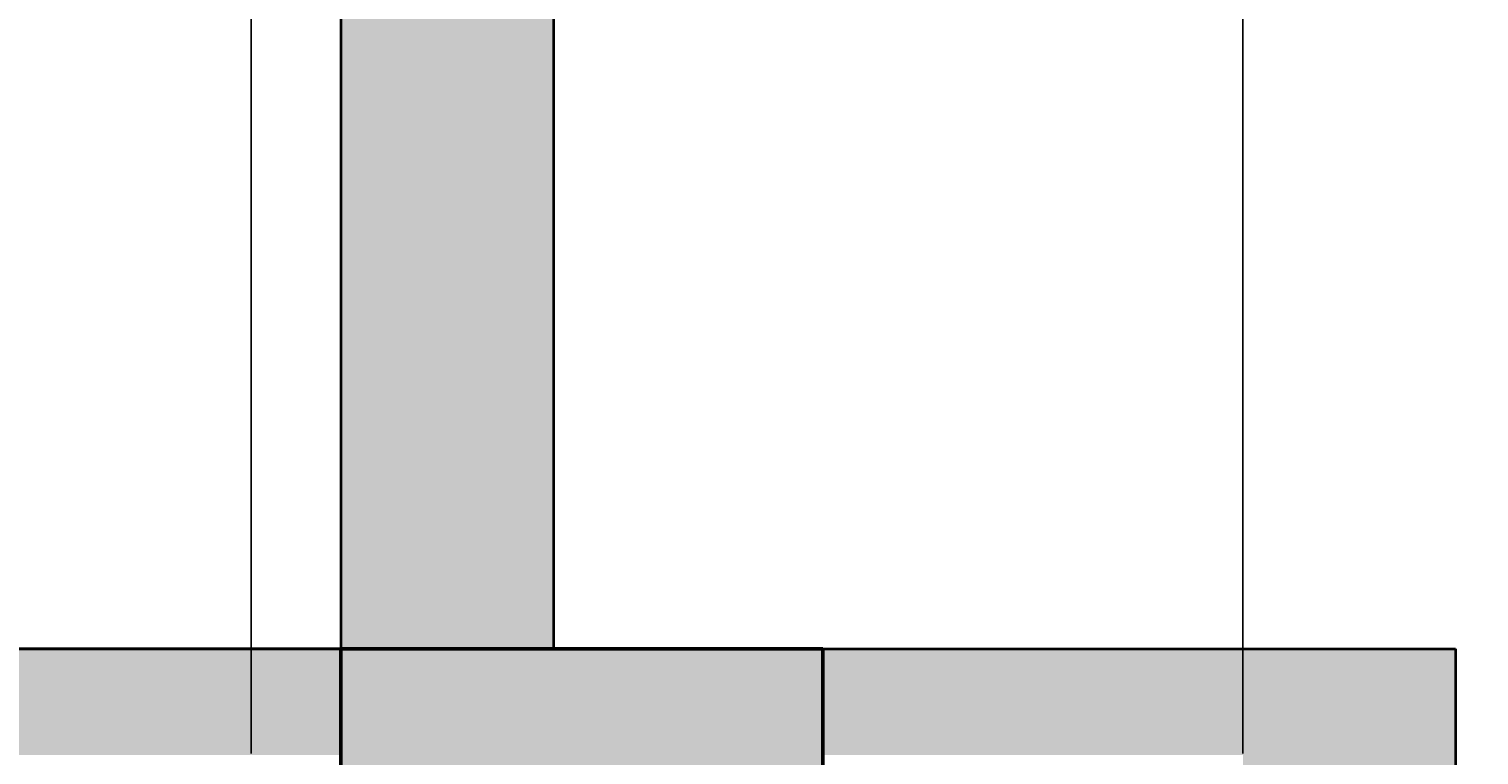
# Model space of a CAD drawing. Units: inches. Extents: x 1998 to 2588, y 1139 to 1977.
# Tile 130 of 134: x 2489 to 2550, y 1637 to 1667. Entities that reach past the tile are written whole.
import ezdxf

# ---------------------------------------------------------------- set-up
doc = ezdxf.new("R2010")
doc.units = ezdxf.units.IN
for name, color, linetype, lineweight in [('A-ANNO-DIMS', 2, 'Continuous', 18), ('A-COLS-PATT', 250, 'Continuous', 13), ('A-WALL-PATT', 252, 'Continuous', 13), ('COLUMN', 10, 'Continuous', 50), ('WALL', 200, 'Continuous', 35)]:
    doc.layers.add(name, color=color, linetype=linetype, lineweight=lineweight)
doc.styles.get("Standard").update_dxf_attribs({"font": 'arial.ttf'})
doc.dimstyles.get("Standard").update_dxf_attribs({"dimtxt": 0.18, "dimasz": 0.18, "dimexe": 0.18, "dimexo": 0.0625, "dimgap": 0.09, "dimtad": 0, "dimtih": 1, "dimtoh": 1, "dimdec": 4, "dimzin": 0, "dimdsep": 46, "dimtxsty": 'Standard', "dimcen": 0.09, "dimadec": 0, "dimazin": 0, "dimtfac": 1, "dimtdec": 4, "dimtofl": 0, "dimtmove": 0, "dimatfit": 3, "dimfxl": 1, "dimtolj": 1, "dimtzin": 0, "dimarcsym": 0})

# ---------------------------------------------------------------- blocks, each defined once
blk = doc.blocks.new('*D24')
at = {"layer": 'A-ANNO-DIMS', "color": 0, "lineweight": -2, "transparency": 16777216}
for p, q in [((2398.535, 1911.232), (2588.309, 1911.232)), ((2588.129, 1911.052), (2588.129, 1570.164)), ((2588.129, 1228.912), (2588.129, 1569.8)), ((2527.535, 1228.732), (2588.309, 1228.732))]:
    blk.add_line(p, q, dxfattribs=at)
at = {"layer": 'A-ANNO-DIMS', "color": 0, "transparency": 16777216}
for points in [[(2588.099, 1911.052), (2588.159, 1911.052), (2588.129, 1911.232)], [(2588.099, 1228.912), (2588.159, 1228.912), (2588.129, 1228.732)]]:
    blk.add_solid(points, dxfattribs=at)
at = {"layer": 'Defpoints', "color": 0, "transparency": 16777216}
for p in [(2398.473, 1911.232), (2588.129, 1911.232), (2527.473, 1228.732)]:
    blk.add_point(p, dxfattribs=at)
at = {"layer": 'A-ANNO-DIMS', "color": 0, "transparency": 16777216, "insert": (2588.129, 1569.982), "char_height": 0.18, "attachment_point": 5}
blk.add_mtext('\\A1;682.5', dxfattribs=at)
blk = doc.blocks.new('*D31')
at = {"layer": 'A-ANNO-DIMS', "color": 0, "lineweight": -2, "transparency": 16777216}
for p, q in [((2498.179, 1636.795), (2498.179, 1977.362)), ((2498.359, 1977.182), (2518.957, 1977.182)), ((2539.999, 1977.182), (2519.4, 1977.182)), ((2540.179, 1636.795), (2540.179, 1977.362))]:
    blk.add_line(p, q, dxfattribs=at)
at = {"layer": 'A-ANNO-DIMS', "color": 0, "transparency": 16777216}
for points in [[(2498.359, 1977.212), (2498.359, 1977.152), (2498.179, 1977.182)], [(2539.999, 1977.212), (2539.999, 1977.152), (2540.179, 1977.182)]]:
    blk.add_solid(points, dxfattribs=at)
at = {"layer": 'Defpoints', "color": 0, "transparency": 16777216}
for p in [(2540.179, 1977.182), (2498.179, 1636.732), (2540.179, 1636.732)]:
    blk.add_point(p, dxfattribs=at)
at = {"layer": 'A-ANNO-DIMS', "color": 0, "transparency": 16777216, "insert": (2519.179, 1977.182), "char_height": 0.18, "attachment_point": 5}
blk.add_mtext('\\A1;42', dxfattribs=at)

msp = doc.modelspace()

# ---------------------------------------------------------------- hatches: boundary and pattern name
at = {"layer": 'A-COLS-PATT'}
h = msp.add_hatch(color=256, dxfattribs=at)
h.dxf.hatch_style = 1
h.paths.add_polyline_path([(2099.4125, 1888.7324), (2087.9729, 1888.7324), (2087.9729, 1868.3278), (2099.4125, 1868.3278)])
h.paths.add_polyline_path([(2234.4125, 1888.7324), (2222.9729, 1888.7324), (2222.9729, 1868.3278), (2234.4125, 1868.3278)])
h.paths.add_polyline_path([(2341.4729, 1886.637), (2330.0332, 1886.637), (2330.0332, 1866.2324), (2341.4729, 1866.2324)])
h.paths.add_polyline_path([(2507.8006, 1882.7324), (2487.396, 1882.7324), (2487.396, 1871.2927), (2507.8006, 1871.2927)])
h.paths.add_polyline_path([(2510.9729, 1766.672), (2490.5682, 1766.672), (2490.5682, 1755.2324), (2510.9729, 1755.2324)])
h.paths.add_polyline_path([(2345.9729, 1759.7324), (2334.5332, 1759.7324), (2334.5332, 1739.3278), (2345.9729, 1739.3278)])
h.paths.add_polyline_path([(2234.4125, 1774.3318), (2222.9729, 1774.3318), (2222.9729, 1753.9272), (2234.4125, 1753.9272)])
h.paths.add_polyline_path([(2099.4125, 1775.637), (2087.9729, 1775.637), (2087.9729, 1755.2324), (2099.4125, 1755.2324)])
h.paths.add_polyline_path([(2098.0956, 1593.7241), (2077.691, 1593.7241), (2077.691, 1582.2845), (2098.0956, 1582.2845)])
h.paths.add_polyline_path([(2227.4729, 1604.637), (2216.0332, 1604.637), (2216.0332, 1584.2324), (2227.4729, 1584.2324)])
h.paths.add_polyline_path([(2345.9729, 1647.5211), (2334.5332, 1647.5211), (2334.5332, 1627.1165), (2345.9729, 1627.1165)])
h.paths.add_polyline_path([(2522.3775, 1641.2324), (2501.9729, 1641.2324), (2501.9729, 1629.7927), (2522.3775, 1629.7927)])
h.paths.add_polyline_path([(2522.3775, 1480.7324), (2501.9729, 1480.7324), (2501.9729, 1469.2927), (2522.3775, 1469.2927)])
h.paths.add_polyline_path([(2345.9729, 1488.5616), (2334.5332, 1488.5616), (2334.5332, 1468.1569), (2345.9729, 1468.1569)])
h.paths.add_polyline_path([(2234.4125, 1486.137), (2227.4729, 1486.137), (2227.4729, 1465.7324), (2234.4125, 1465.7324)])
h.paths.add_polyline_path([(2227.4729, 1486.137), (2222.9729, 1486.137), (2222.9729, 1465.7324), (2227.4729, 1465.7324)])
h.paths.add_polyline_path([(2108.3775, 1470.2324), (2087.9729, 1470.2324), (2087.9729, 1458.7927), (2108.3775, 1458.7927)])
h.paths.add_polyline_path([(2096.9729, 1365.5012), (2087.9729, 1365.5012), (2087.9729, 1345.0966), (2096.9729, 1345.0966)])
h.paths.add_polyline_path([(2087.9729, 1365.5012), (2085.5332, 1365.5012), (2085.5332, 1345.0966), (2087.9729, 1345.0966)])
h.paths.add_polyline_path([(2234.4125, 1285.137), (2222.9729, 1285.137), (2222.9729, 1264.7324), (2234.4125, 1264.7324)])
h.paths.add_polyline_path([(2345.9729, 1285.137), (2334.5332, 1285.137), (2334.5332, 1264.7324), (2345.9729, 1264.7324)])
h.paths.add_polyline_path([(2503.1458, 1240.172), (2482.7412, 1240.172), (2482.7412, 1228.7324), (2503.1458, 1228.7324)])
h.paths.add_polyline_path([(2510.9729, 1369.172), (2490.5682, 1369.172), (2490.5682, 1357.7324), (2510.9729, 1357.7324)])
at = {"layer": 'A-WALL-PATT'}
h = msp.add_hatch(color=256, dxfattribs=at)
h.dxf.hatch_style = 1
h.paths.add_polyline_path([(2527.4729, 1362.2324), (2510.9729, 1362.2324), (2510.9729, 1357.7324), (2518.4729, 1357.7324), (2518.4729, 1237.7324), (2503.1458, 1237.7324), (2503.1458, 1228.7324), (2527.4729, 1228.7324)])
h.paths.add_polyline_path([(2490.5682, 1362.2324), (2398.4729, 1362.2324), (2398.4729, 1357.7324), (2490.5682, 1357.7324)])
h.paths.add_polyline_path([(2224.9729, 1264.7324), (2222.9729, 1264.7324), (2222.9729, 1232.4125), (2341.4729, 1232.4125), (2341.4729, 1234.4125), (2224.9729, 1234.4125)])
h.paths.add_polyline_path([(2334.5332, 1273.7324), (2264.7638, 1273.7324), (2264.7638, 1269.5611, -0.043659), (2264.3413, 1264.7324), (2334.5332, 1264.7324)])
h.paths.add_polyline_path([(2236.9551, 1273.7324), (2234.4125, 1273.7324), (2234.4125, 1264.7324), (2236.9551, 1264.7324), (2236.9551, 1269.5611)])
h.paths.add_polyline_path([(2222.9729, 1293.2324), (2096.9729, 1293.2324), (2096.9729, 1345.0966), (2087.9729, 1345.0966), (2087.9729, 1284.2324), (2222.9729, 1284.2324), (2222.9729, 1285.137)])
h.paths.add_polyline_path([(2096.9729, 1458.7927), (2087.9729, 1458.7927), (2087.9729, 1417.7324), (2087.9729, 1413.2324), (2096.9729, 1413.2324), (2096.9729, 1417.7324)])
h.paths.add_polyline_path([(2096.9729, 1413.2324), (2087.9729, 1413.2324), (2087.9729, 1365.5012), (2096.9729, 1365.5012), (2096.9729, 1369.3358)])
h.paths.add_polyline_path([(2186.2943, 1417.7324), (2138.6074, 1417.7324), (2096.9729, 1417.7324), (2096.9729, 1413.2324), (2138.6074, 1413.2324), (2186.2943, 1413.2324)])
h.paths.add_polyline_path([(2181.4729, 1465.7324), (2176.9729, 1465.7324), (2176.9729, 1451.6434), (2181.4729, 1451.6434)])
h.paths.add_polyline_path([(2181.4729, 1422.1664), (2176.9729, 1422.1664), (2176.9729, 1417.7324), (2181.4729, 1417.7324)])
h.paths.add_polyline_path([(2063.9729, 1465.7324), (2087.9729, 1465.7324), (2087.9729, 1470.2324), (2059.4729, 1470.2324), (2059.4729, 1413.2324), (2087.9729, 1413.2324), (2087.9729, 1417.7324), (2063.9729, 1417.7324)])
h.paths.add_polyline_path([(2181.4729, 1755.2324), (2176.9729, 1755.2324), (2176.9729, 1748.6798), (2177.0513, 1748.6798), (2181.4729, 1748.6798)])
h.paths.add_polyline_path([(2227.4729, 1707.2324), (2220.4647, 1707.2324), (2220.4647, 1702.7324), (2222.9729, 1702.7324), (2222.9729, 1604.637), (2227.4729, 1604.637)])
h.paths.add_polyline_path([(2114.9729, 1702.7324), (2105.9729, 1702.7324), (2105.9729, 1628.4781, -0.0318759), (2110.1012, 1628.7416), (2114.9729, 1628.7416)])
h.paths.add_polyline_path([(2345.9729, 1739.3278), (2341.4729, 1739.3278), (2341.4729, 1647.5211), (2345.9729, 1647.5211)])
h.paths.add_polyline_path([(2350.6273, 1641.2324), (2345.9729, 1641.2324), (2345.9729, 1636.7324), (2350.6273, 1636.7324), (2350.6273, 1639.8729)])
h.paths.add_polyline_path([(2501.9729, 1641.2324), (2407.9729, 1641.2324), (2392.5005, 1641.2324), (2392.5005, 1639.8729), (2392.5005, 1636.7324), (2501.9729, 1636.7324)])
h.paths.add_polyline_path([(2510.9729, 1755.2324), (2501.9729, 1755.2324), (2501.9729, 1641.2324), (2510.9729, 1641.2324)])
h.paths.add_polyline_path([(2549.1786, 1641.2324), (2522.3775, 1641.2324), (2522.3775, 1636.7324), (2540.1786, 1636.7324), (2540.1786, 1480.7324), (2522.3775, 1480.7324), (2522.3775, 1476.2324), (2549.1786, 1476.2324)])
h.paths.add_polyline_path([(2498.1786, 1594.7324), (2407.9729, 1594.7324), (2407.9729, 1585.7324), (2416.9729, 1585.7324), (2489.1786, 1585.7324), (2489.1786, 1531.7324), (2416.9729, 1531.7324), (2407.9729, 1531.7324), (2407.9729, 1522.7324), (2498.1786, 1522.7324)])
h.paths.add_polyline_path([(2351.6437, 1480.7324), (2345.9729, 1480.7324), (2345.9729, 1476.2324), (2351.6437, 1476.2324), (2351.6437, 1477.5919)])
h.paths.add_polyline_path([(2501.9729, 1480.7324), (2498.1786, 1480.7324), (2407.9729, 1480.7324), (2393.5168, 1480.7324), (2393.5168, 1477.5919), (2393.5168, 1476.2324), (2501.9729, 1476.2324)])

# ---------------------------------------------------------------- linework, layer by layer
at = {"layer": 'COLUMN'}
msp.add_lwpolyline([(2522.3775, 1641.2324), (2522.3775, 1629.7927), (2501.9729, 1629.7927), (2501.9729, 1641.2324)], close=True, dxfattribs=at)
at = {"layer": 'WALL'}
for p, q in [((2501.9729, 1755.2324), (2501.9729, 1641.2324)), ((2510.9729, 1755.2324), (2510.9729, 1641.2324)), ((2501.9729, 1641.2324), (2391.5845, 1641.2324)), ((2407.9729, 1641.2324), (2549.1786, 1641.2324)), ((2549.1786, 1641.2324), (2549.1786, 1476.2324))]:
    msp.add_line(p, q, dxfattribs=at)

# ---------------------------------------------------------------- dimensions: what is measured, and where the dimension line sits
at = {"layer": 'A-ANNO-DIMS'}
dim = msp.add_linear_dim(base=(2540.1786, 1977.1824), p1=(2498.1786, 1636.7324), p2=(2540.1786, 1636.7324), dimstyle='Standard', override={"dimdec": 0, "dimlfac": 1, "dimrnd": 0, "dimzin": 0, "dimdsep": 46, "dimlunit": 2}, dxfattribs=at)
dim.commit()
dim.dimension.update_dxf_attribs({"geometry": '*D31', "text_midpoint": (2519.1786, 1977.1824)})
dim = msp.add_linear_dim(base=(2588.1286, 1911.2324), p1=(2527.4729, 1228.7324), p2=(2398.4729, 1911.2324), angle=90, dimstyle='Standard', override={"dimdec": 1, "dimlfac": 1, "dimrnd": 0, "dimzin": 0, "dimdsep": 46, "dimlunit": 2}, dxfattribs=at)
dim.commit()
dim.dimension.update_dxf_attribs({"geometry": '*D24', "text_midpoint": (2588.1286, 1569.9824)})

doc.saveas('drawing.dxf')
